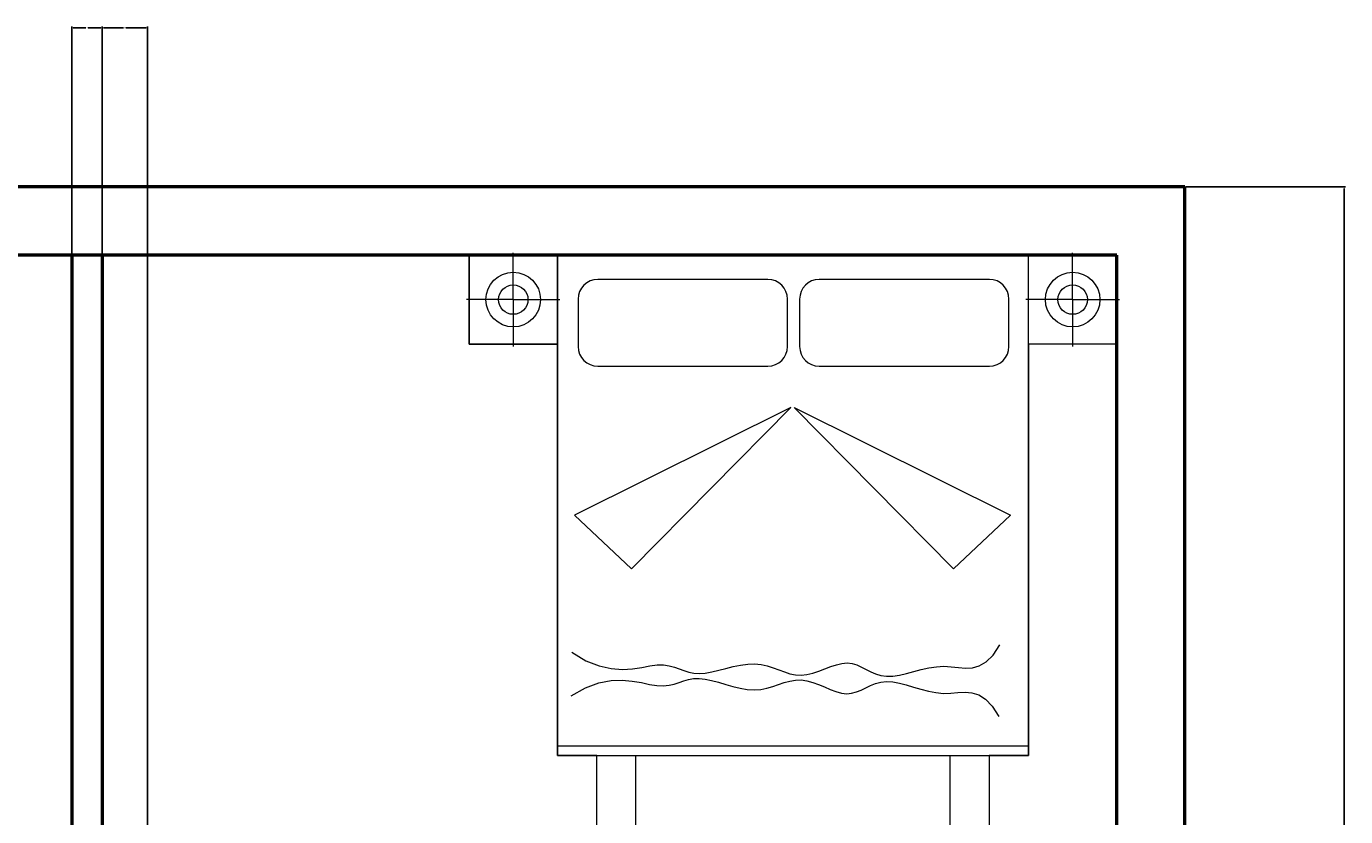
# Model space of a CAD drawing. Units: inches. Extents: x 1798 to 2141, y 1923 to 2386.
# Tile 9 of 9: x 1967 to 2141, y 2281 to 2386. Entities that reach past the tile are written whole.
import ezdxf

# ---------------------------------------------------------------- set-up
doc = ezdxf.new("R2010")
doc.units = ezdxf.units.IN
for name, color, linetype, lineweight in [('A-ANNO-DIMS', 2, 'Continuous', 18), ('A-FURN', 8, 'Continuous', 13), ('wall', 4, 'Continuous', 50)]:
    doc.layers.add(name, color=color, linetype=linetype, lineweight=lineweight)
doc.styles.get("Standard").update_dxf_attribs({"font": 'arial.ttf'})
doc.dimstyles.get("Standard").update_dxf_attribs({"dimtxt": 0.18, "dimasz": 0.18, "dimexe": 0.18, "dimexo": 0.0625, "dimgap": 0.09, "dimtad": 0, "dimtih": 1, "dimtoh": 1, "dimdec": 4, "dimzin": 0, "dimdsep": 46, "dimtxsty": 'Standard', "dimcen": 0.09, "dimadec": 0, "dimazin": 0, "dimtfac": 1, "dimtdec": 4, "dimtofl": 0, "dimtmove": 0, "dimatfit": 3, "dimfxl": 1, "dimtolj": 1, "dimtzin": 0, "dimarcsym": 0})

# ---------------------------------------------------------------- blocks, each defined once
blk = doc.blocks.new('A$C4F543DC7')
for p, q in [((0.0134, 3.35, -0.1688), (3.3134, 3.35, -0.1688)), ((0.4634, 3.35, -0.1688), (0.0134, 3.35, -0.1688)), ((0.0134, 2.896, -0.1688), (0.0134, 3.35, -0.1688)), ((0.0134, 3.35, -0.1688), (0.0134, 2.896, -0.1688)), ((0.2381, 3.1233, -0.4388), (0.2381, 3.3614, -0.4388)), ((0.4634, 3.35, -0.1688), (0.4634, 0.8, -0.1688)), ((2.8634, 3.35, -0.1688), (0.4634, 3.35, -0.1688)), ((0.4634, 2.896, -0.1688), (0.4634, 3.35, -0.1688)), ((2.8634, 0.8, -0.1688), (2.8634, 3.35, -0.1688)), ((2.8634, 3.35, -0.1688), (3.3134, 3.35, -0.1688)), ((2.8634, 2.896, -0.1688), (2.8634, 3.35, -0.1688)), ((3.0888, 3.1233, -0.4388), (3.0888, 3.3614, -0.4388)), ((3.3134, 3.35, -0.1688), (3.3134, 2.896, -0.1688)), ((3.3134, 3.35, -0.1688), (3.3134, 2.896, -0.1688)), ((1.5354, 3.226, -0.1688), (0.6684, 3.226, -0.1688)), ((2.6644, 3.226, -0.1688), (1.7974, 3.226, -0.1688)), ((0.2381, 3.1233, -0.4388), (0, 3.1233, -0.4388)), ((0.2381, 3.1233, -0.4388), (0.4762, 3.1233, -0.4388)), ((0.2381, 3.1233, -0.4388), (0.2381, 2.8852, -0.4388)), ((0.5684, 3.126, -0.1688), (0.5684, 2.884, -0.1688)), ((1.6354, 2.884, -0.1688), (1.6354, 3.126, -0.1688)), ((1.6974, 3.126, -0.1688), (1.6974, 2.884, -0.1688)), ((2.7644, 2.884, -0.1688), (2.7644, 3.126, -0.1688)), ((3.0888, 3.1233, -0.4388), (2.8507, 3.1233, -0.4388)), ((3.0888, 3.1233, -0.4388), (3.0888, 2.8852, -0.4388)), ((3.0888, 3.1233, -0.4388), (3.3269, 3.1233, -0.4388)), ((0.4634, 2.896, -0.1688), (0.0134, 2.896, -0.1688)), ((0.0134, 2.896, -0.1688), (0.4634, 2.896, -0.1688)), ((0.4634, 0.8, -0.1688), (0.4634, 2.896, -0.1688)), ((2.8634, 2.896, -0.1688), (2.8634, 0.8, -0.1688)), ((3.3134, 2.896, -0.1688), (2.8634, 2.896, -0.1688)), ((3.3134, 2.896, -0.1688), (2.8634, 2.896, -0.1688)), ((0.6684, 2.784, -0.1688), (1.5354, 2.784, -0.1688)), ((1.7974, 2.784, -0.1688), (2.6644, 2.784, -0.1688)), ((1.6534, 2.573, -0.1688), (0.5504, 2.025, -0.1688)), ((0.8414, 1.752, -0.1688), (1.6534, 2.573, -0.1688)), ((2.4814, 1.752, -0.1688), (1.6694, 2.573, -0.1688)), ((1.6694, 2.573, -0.1688), (2.7724, 2.025, -0.1688)), ((0.5504, 2.025, -0.1688), (0.8414, 1.752, -0.1688)), ((2.7724, 2.025, -0.1688), (2.4814, 1.752, -0.1688)), ((2.683, 1.312, -0.1688), (2.7182, 1.3641, -0.1688)), ((0.5369, 1.3267, -0.1688), (0.6088, 1.2835, -0.1688)), ((0.6088, 1.2835, -0.1688), (0.6756, 1.2566, -0.1688)), ((2.6479, 1.2774, -0.1688), (2.683, 1.312, -0.1688)), ((0.6756, 1.2566, -0.1688), (0.7373, 1.2428, -0.1688)), ((0.7373, 1.2428, -0.1688), (0.794, 1.239, -0.1688)), ((0.794, 1.239, -0.1688), (0.8457, 1.242, -0.1688)), ((0.8457, 1.242, -0.1688), (0.8925, 1.2489, -0.1688)), ((0.8925, 1.2489, -0.1688), (0.9345, 1.2564, -0.1688)), ((0.9345, 1.2564, -0.1688), (0.9718, 1.2615, -0.1688)), ((0.9718, 1.2615, -0.1688), (1.0044, 1.2617, -0.1688)), ((1.0044, 1.2617, -0.1688), (1.0334, 1.2578, -0.1688)), ((1.0334, 1.2578, -0.1688), (1.0597, 1.2509, -0.1688)), ((1.0597, 1.2509, -0.1688), (1.0842, 1.2424, -0.1688)), ((1.0842, 1.2424, -0.1688), (1.1081, 1.2336, -0.1688)), ((1.1081, 1.2336, -0.1688), (1.1322, 1.2257, -0.1688)), ((1.1322, 1.2257, -0.1688), (1.1577, 1.2201, -0.1688)), ((1.1577, 1.2201, -0.1688), (1.1855, 1.218, -0.1688)), ((1.1855, 1.218, -0.1688), (1.2163, 1.2204, -0.1688)), ((1.2163, 1.2204, -0.1688), (1.2498, 1.2264, -0.1688)), ((1.2498, 1.2264, -0.1688), (1.2852, 1.2347, -0.1688)), ((1.2852, 1.2347, -0.1688), (1.3218, 1.2441, -0.1688)), ((1.3218, 1.2441, -0.1688), (1.3591, 1.2533, -0.1688)), ((1.3591, 1.2533, -0.1688), (1.3963, 1.2612, -0.1688)), ((1.3963, 1.2612, -0.1688), (1.4328, 1.2664, -0.1688)), ((1.4328, 1.2664, -0.1688), (1.4679, 1.2677, -0.1688)), ((1.4679, 1.2677, -0.1688), (1.501, 1.2643, -0.1688)), ((1.501, 1.2643, -0.1688), (1.5324, 1.257, -0.1688)), ((1.5324, 1.257, -0.1688), (1.5624, 1.2473, -0.1688)), ((1.5624, 1.2473, -0.1688), (1.5915, 1.2365, -0.1688)), ((1.5915, 1.2365, -0.1688), (1.6199, 1.2259, -0.1688)), ((1.6199, 1.2259, -0.1688), (1.6481, 1.2169, -0.1688)), ((1.6481, 1.2169, -0.1688), (1.6765, 1.2108, -0.1688)), ((1.6765, 1.2108, -0.1688), (1.7053, 1.209, -0.1688)), ((1.7053, 1.209, -0.1688), (1.7349, 1.2124, -0.1688)), ((1.7349, 1.2124, -0.1688), (1.7651, 1.2199, -0.1688)), ((1.7651, 1.2199, -0.1688), (1.7955, 1.2301, -0.1688)), ((1.7955, 1.2301, -0.1688), (1.8258, 1.2417, -0.1688)), ((1.8258, 1.2417, -0.1688), (1.8557, 1.2531, -0.1688)), ((1.8557, 1.2531, -0.1688), (1.8849, 1.263, -0.1688)), ((1.8849, 1.263, -0.1688), (1.913, 1.2698, -0.1688)), ((1.913, 1.2698, -0.1688), (1.9397, 1.2722, -0.1688)), ((1.9397, 1.2722, -0.1688), (1.9649, 1.2692, -0.1688)), ((1.9649, 1.2692, -0.1688), (1.989, 1.2617, -0.1688)), ((1.989, 1.2617, -0.1688), (2.0124, 1.2512, -0.1688)), ((2.0124, 1.2512, -0.1688), (2.0359, 1.2391, -0.1688)), ((2.0359, 1.2391, -0.1688), (2.0599, 1.2269, -0.1688)), ((2.0599, 1.2269, -0.1688), (2.0849, 1.216, -0.1688)), ((2.0849, 1.216, -0.1688), (2.1117, 1.2077, -0.1688)), ((2.2062, 1.21, -0.1688), (2.242, 1.2182, -0.1688)), ((2.242, 1.2182, -0.1688), (2.2791, 1.2279, -0.1688)), ((2.2791, 1.2279, -0.1688), (2.3173, 1.2378, -0.1688)), ((2.3173, 1.2378, -0.1688), (2.3558, 1.2465, -0.1688)), ((2.3558, 1.2465, -0.1688), (2.3944, 1.2527, -0.1688)), ((2.3944, 1.2527, -0.1688), (2.4325, 1.255, -0.1688)), ((2.4325, 1.255, -0.1688), (2.4698, 1.2529, -0.1688)), ((2.4698, 1.2529, -0.1688), (2.5064, 1.2488, -0.1688)), ((2.5064, 1.2488, -0.1688), (2.5423, 1.2459, -0.1688)), ((2.5423, 1.2459, -0.1688), (2.5777, 1.2476, -0.1688)), ((2.5777, 1.2476, -0.1688), (2.6129, 1.257, -0.1688)), ((2.6129, 1.257, -0.1688), (2.6479, 1.2774, -0.1688)), ((0.5334, 1.105, -0.1688), (0.6067, 1.1458, -0.1688)), ((0.6067, 1.1458, -0.1688), (0.6743, 1.1706, -0.1688)), ((0.6743, 1.1706, -0.1688), (0.7364, 1.1825, -0.1688)), ((0.7364, 1.1825, -0.1688), (0.7931, 1.1846, -0.1688)), ((0.7931, 1.1846, -0.1688), (0.8447, 1.1799, -0.1688)), ((0.8447, 1.1799, -0.1688), (0.8913, 1.1716, -0.1688)), ((0.8913, 1.1716, -0.1688), (0.9331, 1.1628, -0.1688)), ((0.9331, 1.1628, -0.1688), (0.9701, 1.1565, -0.1688)), ((0.9701, 1.1565, -0.1688), (1.0027, 1.1552, -0.1688)), ((1.0027, 1.1552, -0.1688), (1.0318, 1.1582, -0.1688)), ((1.0318, 1.1582, -0.1688), (1.0583, 1.1642, -0.1688)), ((1.0583, 1.1642, -0.1688), (1.0831, 1.172, -0.1688)), ((1.0831, 1.172, -0.1688), (1.1072, 1.18, -0.1688)), ((1.1072, 1.18, -0.1688), (1.1316, 1.1872, -0.1688)), ((1.1316, 1.1872, -0.1688), (1.1573, 1.192, -0.1688)), ((1.1573, 1.192, -0.1688), (1.1851, 1.1932, -0.1688)), ((1.1851, 1.1932, -0.1688), (1.2158, 1.1898, -0.1688)), ((1.2158, 1.1898, -0.1688), (1.2491, 1.1828, -0.1688)), ((1.2491, 1.1828, -0.1688), (1.2842, 1.1734, -0.1688)), ((1.2842, 1.1734, -0.1688), (1.3206, 1.1629, -0.1688)), ((1.3206, 1.1629, -0.1688), (1.3575, 1.1524, -0.1688)), ((1.3575, 1.1524, -0.1688), (1.3945, 1.1434, -0.1688)), ((1.3945, 1.1434, -0.1688), (1.4308, 1.1371, -0.1688)), ((1.499, 1.137, -0.1688), (1.5306, 1.1433, -0.1688)), ((1.5306, 1.1433, -0.1688), (1.5609, 1.152, -0.1688)), ((1.5609, 1.152, -0.1688), (1.5903, 1.1619, -0.1688)), ((1.5903, 1.1619, -0.1688), (1.6191, 1.1716, -0.1688)), ((1.6191, 1.1716, -0.1688), (1.6475, 1.1797, -0.1688)), ((1.6475, 1.1797, -0.1688), (1.676, 1.1849, -0.1688)), ((1.676, 1.1849, -0.1688), (1.7049, 1.1858, -0.1688)), ((1.7049, 1.1858, -0.1688), (1.7344, 1.1816, -0.1688)), ((1.7344, 1.1816, -0.1688), (1.7643, 1.1731, -0.1688)), ((1.7643, 1.1731, -0.1688), (1.7944, 1.1619, -0.1688)), ((1.7944, 1.1619, -0.1688), (1.8244, 1.1494, -0.1688)), ((1.8244, 1.1494, -0.1688), (1.8539, 1.137, -0.1688)), ((2.0106, 1.134, -0.1688), (2.0344, 1.1454, -0.1688)), ((2.0344, 1.1454, -0.1688), (2.0588, 1.1568, -0.1688)), ((2.0588, 1.1568, -0.1688), (2.0842, 1.167, -0.1688)), ((2.0842, 1.167, -0.1688), (2.1112, 1.1743, -0.1688)), ((2.1112, 1.1743, -0.1688), (2.1403, 1.1775, -0.1688)), ((2.1117, 1.2077, -0.1688), (2.1407, 1.2037, -0.1688)), ((2.1403, 1.1775, -0.1688), (2.1718, 1.1755, -0.1688)), ((2.1407, 1.2037, -0.1688), (2.1723, 1.2047, -0.1688)), ((2.1718, 1.1755, -0.1688), (2.2056, 1.1691, -0.1688)), ((2.1723, 1.2047, -0.1688), (2.2062, 1.21, -0.1688)), ((2.2056, 1.1691, -0.1688), (2.2411, 1.1598, -0.1688)), ((2.2411, 1.1598, -0.1688), (2.2779, 1.1489, -0.1688)), ((2.2779, 1.1489, -0.1688), (2.3157, 1.1379, -0.1688)), ((1.4308, 1.1371, -0.1688), (1.4658, 1.1347, -0.1688)), ((1.4658, 1.1347, -0.1688), (1.499, 1.137, -0.1688)), ((1.8539, 1.137, -0.1688), (1.8827, 1.1263, -0.1688)), ((1.8827, 1.1263, -0.1688), (1.9106, 1.1186, -0.1688)), ((1.9106, 1.1186, -0.1688), (1.9373, 1.1153, -0.1688)), ((1.9373, 1.1153, -0.1688), (1.9625, 1.1176, -0.1688)), ((1.9625, 1.1176, -0.1688), (1.9868, 1.1243, -0.1688)), ((1.9868, 1.1243, -0.1688), (2.0106, 1.134, -0.1688)), ((2.3157, 1.1379, -0.1688), (2.354, 1.1279, -0.1688)), ((2.354, 1.1279, -0.1688), (2.3923, 1.1205, -0.1688)), ((2.3923, 1.1205, -0.1688), (2.4304, 1.117, -0.1688)), ((2.4304, 1.117, -0.1688), (2.4677, 1.118, -0.1688)), ((2.4677, 1.118, -0.1688), (2.5043, 1.1209, -0.1688)), ((2.5043, 1.1209, -0.1688), (2.5403, 1.1226, -0.1688)), ((2.5403, 1.1226, -0.1688), (2.5757, 1.1199, -0.1688)), ((2.5757, 1.1199, -0.1688), (2.6106, 1.1094, -0.1688)), ((2.6106, 1.1094, -0.1688), (2.645, 1.0879, -0.1688)), ((2.645, 1.0879, -0.1688), (2.6789, 1.0522, -0.1688)), ((2.6789, 1.0522, -0.1688), (2.7124, 0.999, -0.1688)), ((0.4634, 0.85, -0.1688), (2.8634, 0.85, -0.1688)), ((0.4634, 0.8, -0.1688), (2.8634, 0.8, -0.1688)), ((0.6634, 0.8, -0.1688), (0.4634, 0.8, -0.1688)), ((0.6634, 0.8, -0.1688), (2.6634, 0.8, -0.1688)), ((0.6634, 0.104, -0.1688), (0.6634, 0.8, -0.1688)), ((0.6634, 0.104, -0.1688), (0.6634, 0.8, -0.1688)), ((0.8634, 0.281, -0.1688), (0.8634, 0.8, -0.1688)), ((2.4634, 0.8, -0.1688), (2.4634, 0.281, -0.1688)), ((2.8634, 0.8, -0.1688), (2.6634, 0.8, -0.1688)), ((2.6634, 0.8, -0.1688), (2.6634, 0.104, -0.1688)), ((2.6634, 0.8, -0.1688), (2.6634, 0.104, -0.1688))]:
    blk.add_line(p, q)
for centre, radius in [((0.2381, 3.1233, -0.4388), 0.139), ((3.0888, 3.1233, -0.4388), 0.139), ((0.2381, 3.1233, -0.4388), 0.075), ((3.0888, 3.1233, -0.4388), 0.075)]:
    blk.add_circle(centre, radius)
for centre, radius, start, end in [((0.6684, 3.126, -0.1688), 0.1, 90, 180), ((1.5354, 3.126, -0.1688), 0.1, 0, 90), ((1.7974, 3.126, -0.1688), 0.1, 90, 180), ((2.6644, 3.126, -0.1688), 0.1, 0, 90), ((0.6684, 2.884, -0.1688), 0.1, 180, 270), ((1.5354, 2.884, -0.1688), 0.1, 270, 0), ((1.7974, 2.884, -0.1688), 0.1, 180, 270), ((2.6644, 2.884, -0.1688), 0.1, 270, 0), ((0.6994, 0.3472, -0.1688), 0.1769, 258.2616, 338.03196), ((2.6275, 0.3472, -0.1688), 0.1769, 201.96804, 281.7384), ((1.6634, 4.8597, -0.1688), 4.8597, 258.12517, 281.87483), ((1.6634, 4.8597, -0.1688), 4.8597, 258.12517, 281.87483)]:
    blk.add_arc(centre, radius, start, end)
blk = doc.blocks.new('*D32')
at = {"layer": 'A-ANNO-DIMS', "color": 0, "lineweight": -2, "transparency": 16777216}
for p, q in [((2119.58, 2364.32), (2140.72, 2364.32)), ((2140.54, 2364.14), (2140.54, 2154.51)), ((2140.54, 1944.5), (2140.54, 2154.14)), ((2119.58, 1944.32), (2140.72, 1944.32))]:
    blk.add_line(p, q, dxfattribs=at)
at = {"layer": 'A-ANNO-DIMS', "color": 0, "transparency": 16777216}
for points in [[(2140.51, 2364.14), (2140.57, 2364.14), (2140.54, 2364.32)], [(2140.51, 1944.5), (2140.57, 1944.5), (2140.54, 1944.32)]]:
    blk.add_solid(points, dxfattribs=at)
at = {"layer": 'Defpoints', "color": 0, "transparency": 16777216}
for p in [(2119.51, 2364.32), (2140.54, 2364.32), (2119.51, 1944.32)]:
    blk.add_point(p, dxfattribs=at)
at = {"layer": 'A-ANNO-DIMS', "color": 0, "transparency": 16777216, "insert": (2140.54, 2154.32), "char_height": 0.18, "attachment_point": 5}
blk.add_mtext('\\A1;420', dxfattribs=at)
blk = doc.blocks.new('*D34')
at = {"layer": 'A-ANNO-DIMS', "color": 0, "lineweight": -2, "transparency": 16777216}
for p, q in [((1972.51, 2355.39), (1972.51, 2385.53)), ((1972.69, 2385.35), (1974.36, 2385.35)), ((1976.33, 2385.35), (1974.67, 2385.35)), ((1976.51, 2355.39), (1976.51, 2385.53))]:
    blk.add_line(p, q, dxfattribs=at)
at = {"layer": 'A-ANNO-DIMS', "color": 0, "transparency": 16777216}
for points in [[(1972.69, 2385.38), (1972.69, 2385.32), (1972.51, 2385.35)], [(1976.33, 2385.38), (1976.33, 2385.32), (1976.51, 2385.35)]]:
    blk.add_solid(points, dxfattribs=at)
at = {"layer": 'Defpoints', "color": 0, "transparency": 16777216}
for p in [(1976.51, 2385.35), (1972.51, 2355.32), (1976.51, 2355.32)]:
    blk.add_point(p, dxfattribs=at)
at = {"layer": 'A-ANNO-DIMS', "color": 0, "transparency": 16777216, "insert": (1974.51, 2385.35), "char_height": 0.18, "attachment_point": 5}
blk.add_mtext('\\A1;4', dxfattribs=at)
blk = doc.blocks.new('*D39')
at = {"layer": 'A-ANNO-DIMS', "color": 0, "lineweight": -2, "transparency": 16777216}
for p, q in [((1976.51, 2035.39), (1976.51, 2385.53)), ((1976.69, 2385.35), (1979.36, 2385.35)), ((1982.33, 2385.35), (1979.66, 2385.35)), ((1982.51, 2035.39), (1982.51, 2385.53))]:
    blk.add_line(p, q, dxfattribs=at)
at = {"layer": 'A-ANNO-DIMS', "color": 0, "transparency": 16777216}
for points in [[(1976.69, 2385.38), (1976.69, 2385.32), (1976.51, 2385.35)], [(1982.33, 2385.38), (1982.33, 2385.32), (1982.51, 2385.35)]]:
    blk.add_solid(points, dxfattribs=at)
at = {"layer": 'Defpoints', "color": 0, "transparency": 16777216}
for p in [(1982.51, 2385.35), (1976.51, 2035.32), (1982.51, 2035.32)]:
    blk.add_point(p, dxfattribs=at)
at = {"layer": 'A-ANNO-DIMS', "color": 0, "transparency": 16777216, "insert": (1979.51, 2385.35), "char_height": 0.18, "attachment_point": 5}
blk.add_mtext('\\A1;6', dxfattribs=at)

msp = doc.modelspace()

# ---------------------------------------------------------------- linework, layer by layer
at = {"layer": 'wall'}
for p, q in [((2119.5141, 2364.3239), (1819.5141, 2364.3239)), ((2119.5141, 1944.3239), (2119.5141, 2364.3239)), ((2110.5141, 2355.3239), (1828.5141, 2355.3239)), ((1972.5141, 2355.3239), (1972.5141, 2235.3239)), ((1976.5141, 2355.3239), (1976.5141, 2235.3239)), ((2110.5141, 1944.3239), (2110.5141, 2355.3239))]:
    msp.add_line(p, q, dxfattribs=at)

# ---------------------------------------------------------------- block references
at = {"layer": 'A-FURN', "xscale": 25.91562772622874, "yscale": 25.91562772622874, "zscale": 25.91562772622874}
msp.add_blockref('A$C4F543DC7', (2024.6443, 2268.5065, 4.3733), dxfattribs=at)

# ---------------------------------------------------------------- dimensions: what is measured, and where the dimension line sits
at = {"layer": 'A-ANNO-DIMS'}
for base, p1, p2, picture, middle in [((1976.5141, 2385.3489), (1972.5141, 2355.3239), (1976.5141, 2355.3239), '*D34', (1974.5141, 2385.3489)), ((1982.5141, 2385.3489), (1976.5141, 2035.3239), (1982.5141, 2035.3239), '*D39', (1979.5141, 2385.3489))]:
    dim = msp.add_linear_dim(base=base, p1=p1, p2=p2, dimstyle='Standard', override={"dimdec": 0, "dimlfac": 1, "dimrnd": 0, "dimzin": 0, "dimdsep": 46, "dimlunit": 2}, dxfattribs=at)
    dim.commit()
    dim.dimension.update_dxf_attribs({"geometry": picture, "text_midpoint": middle})
dim = msp.add_linear_dim(base=(2140.5391, 2364.3239), p1=(2119.5141, 1944.3239), p2=(2119.5141, 2364.3239), angle=90, dimstyle='Standard', override={"dimdec": 0, "dimlfac": 1, "dimrnd": 0, "dimzin": 0, "dimdsep": 46, "dimlunit": 2}, dxfattribs=at)
dim.commit()
dim.dimension.update_dxf_attribs({"geometry": '*D32', "text_midpoint": (2140.5391, 2154.3239)})

doc.saveas('drawing.dxf')
